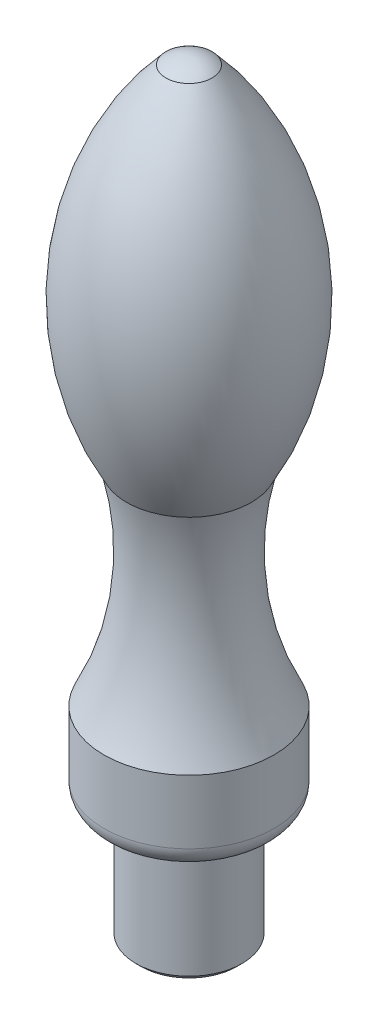
ISO-10303-21;
HEADER;
FILE_DESCRIPTION(('STEP AP214'),'2;1');
FILE_NAME('part.step','',(''),(''),'','','');
FILE_SCHEMA(('AUTOMOTIVE_DESIGN { 1 0 10303 214 1 1 1 1 }'));
ENDSEC;
DATA;
#1=APPLICATION_CONTEXT('core data for automotive mechanical design processes');
#2=APPLICATION_PROTOCOL_DEFINITION('international standard','automotive_design',2000,#1);
#3=PRODUCT_CONTEXT('',#1,'mechanical');
#4=PRODUCT('Part','Part','',(#3));
#5=PRODUCT_RELATED_PRODUCT_CATEGORY('part','',(#4));
#6=PRODUCT_DEFINITION_FORMATION('','',#4);
#7=PRODUCT_DEFINITION_CONTEXT('part definition',#1,'design');
#8=PRODUCT_DEFINITION('design','',#6,#7);
#9=PRODUCT_DEFINITION_SHAPE('','',#8);
#10=(LENGTH_UNIT() NAMED_UNIT(*) SI_UNIT(.MILLI.,.METRE.));
#11=(NAMED_UNIT(*) PLANE_ANGLE_UNIT() SI_UNIT($,.RADIAN.));
#12=(NAMED_UNIT(*) SI_UNIT($,.STERADIAN.) SOLID_ANGLE_UNIT());
#13=UNCERTAINTY_MEASURE_WITH_UNIT(LENGTH_MEASURE(1.E-05),#10,'distance_accuracy_value','');
#14=(GEOMETRIC_REPRESENTATION_CONTEXT(3) GLOBAL_UNCERTAINTY_ASSIGNED_CONTEXT((#13)) GLOBAL_UNIT_ASSIGNED_CONTEXT((#10,
#11,#12)) REPRESENTATION_CONTEXT('',''));
#15=CARTESIAN_POINT('',(0.,0.,0.));
#16=DIRECTION('',(0.,0.,1.));
#17=DIRECTION('',(1.,0.,0.));
#18=AXIS2_PLACEMENT_3D('',#15,#16,#17);
#19=CARTESIAN_POINT('',(0.,11.,0.));
#20=DIRECTION('',(0.,-1.,0.));
#21=DIRECTION('',(0.,0.,-1.));
#22=AXIS2_PLACEMENT_3D('',#19,#20,#21);
#23=CYLINDRICAL_SURFACE('',#22,5.);
#24=CARTESIAN_POINT('',(0.,0.5,0.));
#25=DIRECTION('',(0.,1.,0.));
#26=DIRECTION('',(0.,0.,1.));
#27=AXIS2_PLACEMENT_3D('',#24,#25,#26);
#28=CIRCLE('',#27,5.);
#29=CARTESIAN_POINT('',(0.,0.5,5.));
#30=VERTEX_POINT('',#29);
#31=EDGE_CURVE('E57',#30,#30,#28,.T.);
#32=ORIENTED_EDGE('',*,*,#31,.T.);
#33=EDGE_LOOP('',(#32));
#34=FACE_BOUND('',#33,.T.);
#35=CARTESIAN_POINT('',(0.,11.,0.));
#36=DIRECTION('',(0.,1.,0.));
#37=DIRECTION('',(0.,0.,1.));
#38=AXIS2_PLACEMENT_3D('',#35,#36,#37);
#39=CIRCLE('',#38,5.);
#40=CARTESIAN_POINT('',(0.,11.,5.));
#41=VERTEX_POINT('',#40);
#42=EDGE_CURVE('E63',#41,#41,#39,.T.);
#43=ORIENTED_EDGE('',*,*,#42,.F.);
#44=EDGE_LOOP('',(#43));
#45=FACE_BOUND('',#44,.T.);
#46=ADVANCED_FACE('F41',(#34,#45),#23,.T.);
#47=CARTESIAN_POINT('',(0.,0.,0.));
#48=DIRECTION('',(0.,1.,0.));
#49=DIRECTION('',(0.,0.,1.));
#50=AXIS2_PLACEMENT_3D('',#47,#48,#49);
#51=PLANE('',#50);
#52=CARTESIAN_POINT('',(0.,0.,0.));
#53=DIRECTION('',(0.,1.,0.));
#54=DIRECTION('',(0.,0.,1.));
#55=AXIS2_PLACEMENT_3D('',#52,#53,#54);
#56=CIRCLE('',#55,4.5);
#57=CARTESIAN_POINT('',(0.,0.,4.5));
#58=VERTEX_POINT('',#57);
#59=EDGE_CURVE('E55',#58,#58,#56,.F.);
#60=ORIENTED_EDGE('',*,*,#59,.T.);
#61=EDGE_LOOP('',(#60));
#62=FACE_BOUND('',#61,.T.);
#63=ADVANCED_FACE('F95',(#62),#51,.F.);
#64=CARTESIAN_POINT('',(0.,0.5,0.));
#65=DIRECTION('',(0.,1.,0.));
#66=DIRECTION('',(0.,0.,1.));
#67=AXIS2_PLACEMENT_3D('',#64,#65,#66);
#68=CONICAL_SURFACE('',#67,5.,0.78539816339745);
#69=ORIENTED_EDGE('',*,*,#59,.F.);
#70=EDGE_LOOP('',(#69));
#71=FACE_BOUND('',#70,.T.);
#72=ORIENTED_EDGE('',*,*,#31,.F.);
#73=EDGE_LOOP('',(#72));
#74=FACE_BOUND('',#73,.T.);
#75=ADVANCED_FACE('F98',(#71,#74),#68,.T.);
#76=CARTESIAN_POINT('',(0.,19.,0.));
#77=DIRECTION('',(0.,-1.,0.));
#78=DIRECTION('',(0.,0.,-1.));
#79=AXIS2_PLACEMENT_3D('',#76,#77,#78);
#80=CYLINDRICAL_SURFACE('',#79,8.);
#81=CARTESIAN_POINT('',(0.,13.,0.));
#82=DIRECTION('',(0.,1.,0.));
#83=DIRECTION('',(0.,0.,1.));
#84=AXIS2_PLACEMENT_3D('',#81,#82,#83);
#85=CIRCLE('',#84,8.);
#86=CARTESIAN_POINT('',(0.,13.,8.));
#87=VERTEX_POINT('',#86);
#88=EDGE_CURVE('E48',#87,#87,#85,.T.);
#89=ORIENTED_EDGE('',*,*,#88,.T.);
#90=EDGE_LOOP('',(#89));
#91=FACE_BOUND('',#90,.T.);
#92=CARTESIAN_POINT('',(0.,19.,0.));
#93=DIRECTION('',(0.,1.,0.));
#94=DIRECTION('',(0.,0.,1.));
#95=AXIS2_PLACEMENT_3D('',#92,#93,#94);
#96=CIRCLE('',#95,8.);
#97=CARTESIAN_POINT('',(0.,19.,8.));
#98=VERTEX_POINT('',#97);
#99=EDGE_CURVE('E62',#98,#98,#96,.T.);
#100=ORIENTED_EDGE('',*,*,#99,.F.);
#101=EDGE_LOOP('',(#100));
#102=FACE_BOUND('',#101,.T.);
#103=ADVANCED_FACE('F110',(#91,#102),#80,.T.);
#104=CARTESIAN_POINT('',(0.,11.,0.));
#105=DIRECTION('',(0.,1.,0.));
#106=DIRECTION('',(0.,0.,1.));
#107=AXIS2_PLACEMENT_3D('',#104,#105,#106);
#108=PLANE('',#107);
#109=CARTESIAN_POINT('',(0.,11.,0.));
#110=DIRECTION('',(0.,1.,0.));
#111=DIRECTION('',(0.,0.,1.));
#112=AXIS2_PLACEMENT_3D('',#109,#110,#111);
#113=CIRCLE('',#112,6.);
#114=CARTESIAN_POINT('',(0.,11.,6.));
#115=VERTEX_POINT('',#114);
#116=EDGE_CURVE('E10',#115,#115,#113,.F.);
#117=ORIENTED_EDGE('',*,*,#116,.T.);
#118=EDGE_LOOP('',(#117));
#119=FACE_BOUND('',#118,.T.);
#120=ORIENTED_EDGE('',*,*,#42,.T.);
#121=EDGE_LOOP('',(#120));
#122=FACE_BOUND('',#121,.T.);
#123=ADVANCED_FACE('F86',(#119,#122),#108,.F.);
#124=CARTESIAN_POINT('',(0.,13.,0.));
#125=DIRECTION('',(0.,1.,0.));
#126=DIRECTION('',(0.,0.,1.));
#127=AXIS2_PLACEMENT_3D('',#124,#125,#126);
#128=TOROIDAL_SURFACE('',#127,6.,2.);
#129=ORIENTED_EDGE('',*,*,#116,.F.);
#130=EDGE_LOOP('',(#129));
#131=FACE_BOUND('',#130,.T.);
#132=ORIENTED_EDGE('',*,*,#88,.F.);
#133=EDGE_LOOP('',(#132));
#134=FACE_BOUND('',#133,.T.);
#135=ADVANCED_FACE('F43',(#131,#134),#128,.T.);
#136=CARTESIAN_POINT('',(0.,68.4360989680943,0.));
#137=DIRECTION('',(0.,-1.,0.));
#138=DIRECTION('',(-1.,0.,0.));
#139=AXIS2_PLACEMENT_3D('',#136,#137,#138);
#140=SPHERICAL_SURFACE('',#139,3.56390103190566);
#141=CARTESIAN_POINT('',(0.,71.2665828805468,0.));
#142=DIRECTION('',(0.,-1.,0.));
#143=DIRECTION('',(0.,0.,-1.));
#144=AXIS2_PLACEMENT_3D('',#141,#142,#143);
#145=CIRCLE('',#144,2.16558338250138);
#146=CARTESIAN_POINT('',(0.,71.2665828805468,-2.16558338250138));
#147=VERTEX_POINT('',#146);
#148=EDGE_CURVE('E69',#147,#147,#145,.T.);
#149=ORIENTED_EDGE('',*,*,#148,.F.);
#150=EDGE_LOOP('',(#149));
#151=FACE_BOUND('',#150,.T.);
#152=ADVANCED_FACE('F77',(#151),#140,.T.);
#153=CARTESIAN_POINT('',(0.,52.3517300941799,0.));
#154=DIRECTION('',(0.,-1.,0.));
#155=DIRECTION('',(0.,0.,-1.));
#156=AXIS2_PLACEMENT_3D('',#153,#154,#155);
#157=DEGENERATE_TOROIDAL_SURFACE('',#156,18.4797149701519,28.,.F.);
#158=CARTESIAN_POINT('',(0.,38.5211748542442,0.));
#159=DIRECTION('',(0.,-1.,0.));
#160=DIRECTION('',(0.,0.,-1.));
#161=AXIS2_PLACEMENT_3D('',#158,#159,#160);
#162=CIRCLE('',#161,5.86603911048994);
#163=CARTESIAN_POINT('',(0.,38.5211748542442,-5.86603911048994));
#164=VERTEX_POINT('',#163);
#165=EDGE_CURVE('E68',#164,#164,#162,.T.);
#166=ORIENTED_EDGE('',*,*,#165,.F.);
#167=EDGE_LOOP('',(#166));
#168=FACE_BOUND('',#167,.T.);
#169=ORIENTED_EDGE('',*,*,#148,.T.);
#170=EDGE_LOOP('',(#169));
#171=FACE_BOUND('',#170,.T.);
#172=ADVANCED_FACE('F78',(#168,#171),#157,.F.);
#173=CARTESIAN_POINT('',(0.,31.6100737606168,0.));
#174=DIRECTION('',(0.,-1.,0.));
#175=DIRECTION('',(0.,0.,-1.));
#176=AXIS2_PLACEMENT_3D('',#173,#174,#175);
#177=TOROIDAL_SURFACE('',#176,32.9997207934769,28.);
#178=ORIENTED_EDGE('',*,*,#99,.T.);
#179=EDGE_LOOP('',(#178));
#180=FACE_BOUND('',#179,.T.);
#181=ORIENTED_EDGE('',*,*,#165,.T.);
#182=EDGE_LOOP('',(#181));
#183=FACE_BOUND('',#182,.T.);
#184=ADVANCED_FACE('F74',(#180,#183),#177,.F.);
#185=CLOSED_SHELL('',(#46,#63,#75,#103,#123,#135,#152,#172,#184));
#186=MANIFOLD_SOLID_BREP('B2',#185);
#187=ADVANCED_BREP_SHAPE_REPRESENTATION('',(#18,#186),#14);
#188=SHAPE_DEFINITION_REPRESENTATION(#9,#187);
ENDSEC;
END-ISO-10303-21;
